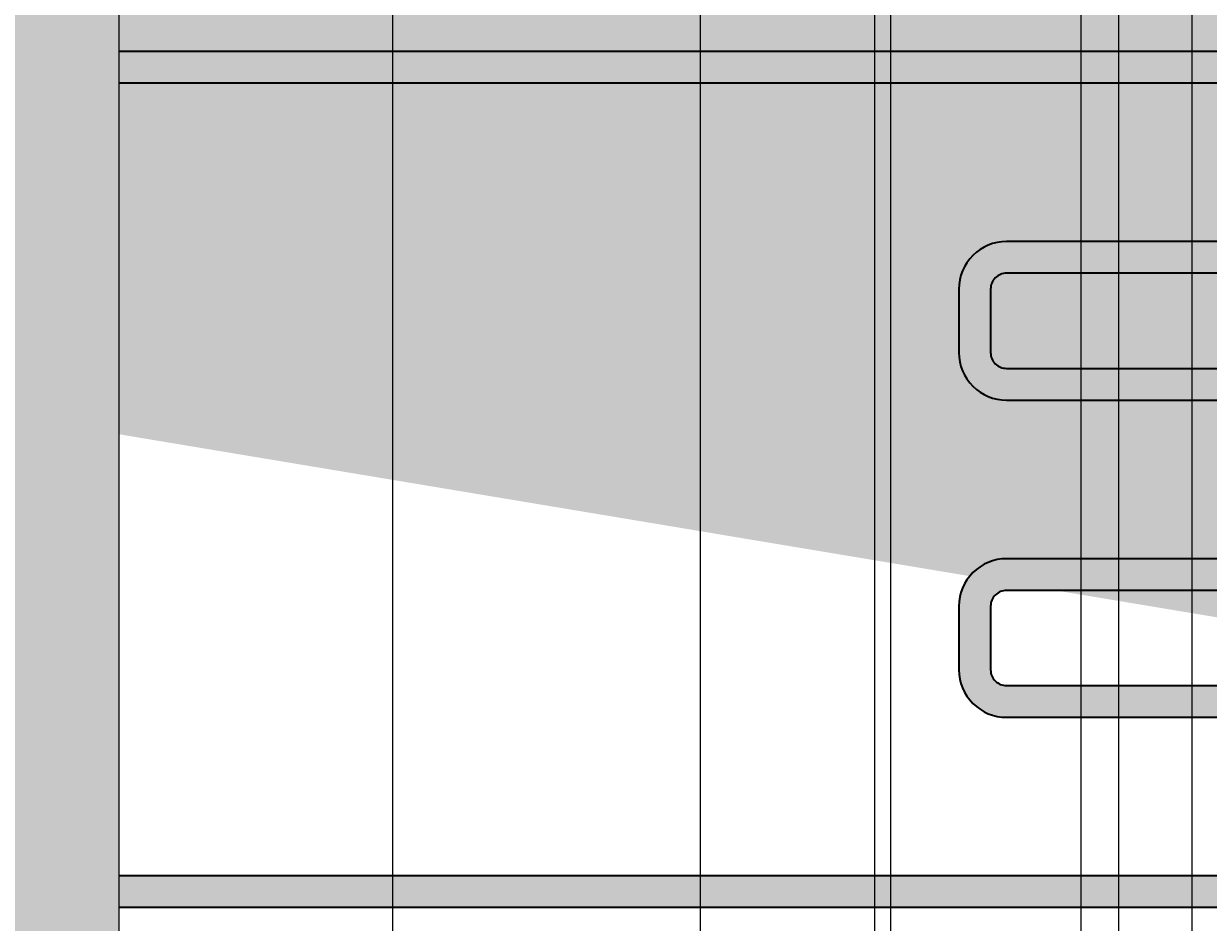
# Model space of a CAD drawing. Units: millimetres. Extents: x -22994 to 29398, y -19990 to 20176.
# Tile 44 of 135: x 99 to 136, y 96 to 124. Entities that reach past the tile are written whole.
import ezdxf

# ---------------------------------------------------------------- set-up
doc = ezdxf.new("R2010")
doc.units = ezdxf.units.MM
doc.header["$MEASUREMENT"] = 0
for name, color, linetype, lineweight in [('M-DIMS', 2, 'Continuous', 18), ('M-EQPM', 7, 'Continuous', 25), ('M-EQPM-PATT', 7, 'Continuous', 18), ('M-PIPE', 7, 'Continuous', 35)]:
    doc.layers.add(name, color=color, linetype=linetype, lineweight=lineweight)
doc.styles.get("Standard").update_dxf_attribs({"font": 'arial.ttf'})
doc.dimstyles.get("Standard").update_dxf_attribs({"dimtxt": 0.18, "dimasz": 10000, "dimexe": 0.18, "dimexo": 0.0625, "dimgap": 0.09, "dimtad": 0, "dimtih": 1, "dimtoh": 1, "dimdec": 0, "dimzin": 0, "dimdsep": 46, "dimtxsty": 'Standard', "dimcen": 0.09, "dimadec": 0, "dimazin": 0, "dimtfac": 1, "dimtdec": 0, "dimtofl": 0, "dimtmove": 0, "dimatfit": 3, "dimfxl": 1, "dimtolj": 1, "dimtzin": 0, "dimlwd": 30, "dimarcsym": 0})

# ---------------------------------------------------------------- blocks, each defined once
blk = doc.blocks.new('*D2')
at = {"layer": 'Defpoints', "color": 0, "transparency": 16777216}
for p in [(6.677, 10.271), (290.852, 10.271), (290.852, -5.079)]:
    blk.add_point(p, dxfattribs=at)
at = {"layer": 'M-DIMS', "color": 0, "lineweight": -2, "transparency": 16777216}
for p, q in [((6.677, 10.209), (6.677, -5.259)), ((290.852, 10.209), (290.852, -5.259))]:
    blk.add_line(p, q, dxfattribs=at)
at = {"layer": 'M-DIMS', "color": 0, "lineweight": 30, "transparency": 16777216}
for p, q in [((-9993.323, -5.079), (-19993.323, -5.079)), ((10290.852, -5.079), (20290.852, -5.079))]:
    blk.add_line(p, q, dxfattribs=at)
at = {"layer": 'M-DIMS', "color": 0, "transparency": 16777216}
for points in [[(-9993.323, 1661.588), (-9993.323, -1671.745), (6.677, -5.079)], [(10290.852, 1661.588), (10290.852, -1671.745), (290.852, -5.079)]]:
    blk.add_solid(points, dxfattribs=at)
at = {"layer": 'M-DIMS', "color": 0, "transparency": 16777216, "insert": (148.765, -5.079), "char_height": 0.18, "attachment_point": 5}
blk.add_mtext('\\A1;284.2', dxfattribs=at)
blk = doc.blocks.new('*D3')
at = {"layer": 'Defpoints', "color": 0, "transparency": 16777216}
for p in [(110.265, 204.165), (110.265, 176.366), (95.833, 127.967)]:
    blk.add_point(p, dxfattribs=at)
at = {"layer": 'M-DIMS', "color": 0, "lineweight": -2, "transparency": 16777216}
for p, q in [((95.833, 128.03), (95.833, 204.345)), ((110.265, 176.429), (110.265, 204.345))]:
    blk.add_line(p, q, dxfattribs=at)
at = {"layer": 'M-DIMS', "color": 0, "lineweight": 30, "transparency": 16777216}
for p, q in [((-9904.167, 204.165), (-19904.167, 204.165)), ((10110.265, 204.165), (20110.265, 204.165))]:
    blk.add_line(p, q, dxfattribs=at)
at = {"layer": 'M-DIMS', "color": 0, "transparency": 16777216}
for points in [[(-9904.167, 1870.832), (-9904.167, -1462.501), (95.833, 204.165)], [(10110.265, 1870.832), (10110.265, -1462.501), (110.265, 204.165)]]:
    blk.add_solid(points, dxfattribs=at)
at = {"layer": 'M-DIMS', "color": 0, "transparency": 16777216, "insert": (103.049, 204.165), "char_height": 0.18, "attachment_point": 5}
blk.add_mtext('\\A1;14.432', dxfattribs=at)
blk = doc.blocks.new('*D4')
at = {"layer": 'Defpoints', "color": 0, "transparency": 16777216}
for p in [(116.265, 204.165), (110.265, 176.366), (116.265, 176.366)]:
    blk.add_point(p, dxfattribs=at)
at = {"layer": 'M-DIMS', "color": 0, "lineweight": -2, "transparency": 16777216}
for p, q in [((110.265, 176.429), (110.265, 204.345)), ((116.265, 176.429), (116.265, 204.345))]:
    blk.add_line(p, q, dxfattribs=at)
at = {"layer": 'M-DIMS', "color": 0, "lineweight": 30, "transparency": 16777216}
for p, q in [((-9889.735, 204.165), (-19889.735, 204.165)), ((10116.265, 204.165), (20116.265, 204.165))]:
    blk.add_line(p, q, dxfattribs=at)
at = {"layer": 'M-DIMS', "color": 0, "transparency": 16777216}
for points in [[(-9889.735, 1870.832), (-9889.735, -1462.501), (110.265, 204.165)], [(10116.265, 1870.832), (10116.265, -1462.501), (116.265, 204.165)]]:
    blk.add_solid(points, dxfattribs=at)
at = {"layer": 'M-DIMS', "color": 0, "transparency": 16777216, "insert": (113.265, 204.165), "char_height": 0.18, "attachment_point": 5}
blk.add_mtext('\\A1;6', dxfattribs=at)
blk = doc.blocks.new('*D5')
at = {"layer": 'Defpoints', "color": 0, "transparency": 16777216}
for p in [(181.265, 204.165), (116.265, 176.366), (181.265, 176.366)]:
    blk.add_point(p, dxfattribs=at)
at = {"layer": 'M-DIMS', "color": 0, "lineweight": -2, "transparency": 16777216}
for p, q in [((116.265, 176.429), (116.265, 204.345)), ((181.265, 176.429), (181.265, 204.345))]:
    blk.add_line(p, q, dxfattribs=at)
at = {"layer": 'M-DIMS', "color": 0, "lineweight": 30, "transparency": 16777216}
for p, q in [((-9883.735, 204.165), (-19883.735, 204.165)), ((10181.265, 204.165), (20181.265, 204.165))]:
    blk.add_line(p, q, dxfattribs=at)
at = {"layer": 'M-DIMS', "color": 0, "transparency": 16777216}
for points in [[(-9883.735, 1870.832), (-9883.735, -1462.501), (116.265, 204.165)], [(10181.265, 1870.832), (10181.265, -1462.501), (181.265, 204.165)]]:
    blk.add_solid(points, dxfattribs=at)
at = {"layer": 'M-DIMS', "color": 0, "transparency": 16777216, "insert": (148.765, 204.165), "char_height": 0.18, "attachment_point": 5}
blk.add_mtext('\\A1;65', dxfattribs=at)
blk = doc.blocks.new('*D6')
at = {"layer": 'Defpoints', "color": 0, "transparency": 16777216}
for p in [(187.265, 204.165), (181.265, 176.366), (187.265, 176.366)]:
    blk.add_point(p, dxfattribs=at)
at = {"layer": 'M-DIMS', "color": 0, "lineweight": -2, "transparency": 16777216}
for p, q in [((181.265, 176.429), (181.265, 204.345)), ((187.265, 176.429), (187.265, 204.345))]:
    blk.add_line(p, q, dxfattribs=at)
at = {"layer": 'M-DIMS', "color": 0, "lineweight": 30, "transparency": 16777216}
for p, q in [((-9818.735, 204.165), (-19818.735, 204.165)), ((10187.265, 204.165), (20187.265, 204.165))]:
    blk.add_line(p, q, dxfattribs=at)
at = {"layer": 'M-DIMS', "color": 0, "transparency": 16777216}
for points in [[(-9818.735, 1870.832), (-9818.735, -1462.501), (181.265, 204.165)], [(10187.265, 1870.832), (10187.265, -1462.501), (187.265, 204.165)]]:
    blk.add_solid(points, dxfattribs=at)
at = {"layer": 'M-DIMS', "color": 0, "transparency": 16777216, "insert": (184.265, 204.165), "char_height": 0.18, "attachment_point": 5}
blk.add_mtext('\\A1;6', dxfattribs=at)
blk = doc.blocks.new('*D7')
at = {"layer": 'Defpoints', "color": 0, "transparency": 16777216}
for p in [(201.697, 204.165), (187.265, 176.366), (201.697, 127.967)]:
    blk.add_point(p, dxfattribs=at)
at = {"layer": 'M-DIMS', "color": 0, "lineweight": -2, "transparency": 16777216}
for p, q in [((187.265, 176.429), (187.265, 204.345)), ((201.697, 128.03), (201.697, 204.345))]:
    blk.add_line(p, q, dxfattribs=at)
at = {"layer": 'M-DIMS', "color": 0, "lineweight": 30, "transparency": 16777216}
for p, q in [((-9812.735, 204.165), (-19812.735, 204.165)), ((10201.697, 204.165), (20201.697, 204.165))]:
    blk.add_line(p, q, dxfattribs=at)
at = {"layer": 'M-DIMS', "color": 0, "transparency": 16777216}
for points in [[(-9812.735, 1870.832), (-9812.735, -1462.501), (187.265, 204.165)], [(10201.697, 1870.832), (10201.697, -1462.501), (201.697, 204.165)]]:
    blk.add_solid(points, dxfattribs=at)
at = {"layer": 'M-DIMS', "color": 0, "transparency": 16777216, "insert": (194.481, 204.165), "char_height": 0.18, "attachment_point": 5}
blk.add_mtext('\\A1;14.432', dxfattribs=at)
blk = doc.blocks.new('*D8')
at = {"layer": 'Defpoints', "color": 0, "transparency": 16777216}
for p in [(227.648, 204.165), (227.648, 146.73), (201.697, 127.967)]:
    blk.add_point(p, dxfattribs=at)
at = {"layer": 'M-DIMS', "color": 0, "lineweight": -2, "transparency": 16777216}
for p, q in [((201.697, 128.03), (201.697, 204.345)), ((227.648, 146.792), (227.648, 204.345))]:
    blk.add_line(p, q, dxfattribs=at)
at = {"layer": 'M-DIMS', "color": 0, "lineweight": 30, "transparency": 16777216}
for p, q in [((-9798.303, 204.165), (-19798.303, 204.165)), ((10227.648, 204.165), (20227.648, 204.165))]:
    blk.add_line(p, q, dxfattribs=at)
at = {"layer": 'M-DIMS', "color": 0, "transparency": 16777216}
for points in [[(-9798.303, 1870.832), (-9798.303, -1462.501), (201.697, 204.165)], [(10227.648, 1870.832), (10227.648, -1462.501), (227.648, 204.165)]]:
    blk.add_solid(points, dxfattribs=at)
at = {"layer": 'M-DIMS', "color": 0, "transparency": 16777216, "insert": (214.673, 204.165), "char_height": 0.18, "attachment_point": 5}
blk.add_mtext('\\A1;25.95', dxfattribs=at)
blk = doc.blocks.new('*D9')
at = {"layer": 'Defpoints', "color": 0, "transparency": 16777216}
for p in [(187.265, 176.366), (306.202, 176.366), (290.852, 10.271)]:
    blk.add_point(p, dxfattribs=at)
at = {"layer": 'M-DIMS', "color": 0, "lineweight": 30, "transparency": 16777216}
for p, q in [((306.202, 10176.366), (306.202, 20176.366)), ((306.202, -9989.729), (306.202, -19989.729))]:
    blk.add_line(p, q, dxfattribs=at)
at = {"layer": 'M-DIMS', "color": 0, "lineweight": -2, "transparency": 16777216}
for p, q in [((187.327, 176.366), (306.382, 176.366)), ((290.915, 10.271), (306.382, 10.271))]:
    blk.add_line(p, q, dxfattribs=at)
at = {"layer": 'M-DIMS', "color": 0, "transparency": 16777216}
for points in [[(-1360.465, 10176.366), (1972.869, 10176.366), (306.202, 176.366)], [(-1360.465, -9989.729), (1972.869, -9989.729), (306.202, 10.271)]]:
    blk.add_solid(points, dxfattribs=at)
at = {"layer": 'M-DIMS', "color": 0, "transparency": 16777216, "insert": (306.202, 93.319), "char_height": 0.18, "attachment_point": 5}
blk.add_mtext('\\A1;166.1', dxfattribs=at)
blk = doc.blocks.new('*D10')
at = {"layer": 'Defpoints', "color": 0, "transparency": 16777216}
for p in [(125.65, 136.071), (133.346, 136.071), (133.346, -5.079)]:
    blk.add_point(p, dxfattribs=at)
at = {"layer": 'M-DIMS', "color": 0, "lineweight": -2, "transparency": 16777216}
for p, q in [((125.65, 136.009), (125.65, -5.259)), ((133.346, 136.009), (133.346, -5.259))]:
    blk.add_line(p, q, dxfattribs=at)
at = {"layer": 'M-DIMS', "color": 0, "lineweight": 30, "transparency": 16777216}
for p, q in [((-9874.35, -5.079), (-19874.35, -5.079)), ((10133.346, -5.079), (20133.346, -5.079))]:
    blk.add_line(p, q, dxfattribs=at)
at = {"layer": 'M-DIMS', "color": 0, "transparency": 16777216}
for points in [[(-9874.35, 1661.588), (-9874.35, -1671.745), (125.65, -5.079)], [(10133.346, 1661.588), (10133.346, -1671.745), (133.346, -5.079)]]:
    blk.add_solid(points, dxfattribs=at)
at = {"layer": 'M-DIMS', "color": 0, "transparency": 16777216, "insert": (129.498, -5.079), "char_height": 0.18, "attachment_point": 5}
blk.add_mtext('\\A1;7.696', dxfattribs=at)
blk = doc.blocks.new('*D11')
at = {"layer": 'Defpoints', "color": 0, "transparency": 16777216}
for p in [(133.346, 136.071), (135.65, 136.071), (135.65, -5.079)]:
    blk.add_point(p, dxfattribs=at)
at = {"layer": 'M-DIMS', "color": 0, "lineweight": -2, "transparency": 16777216}
for p, q in [((133.346, 136.009), (133.346, -5.259)), ((135.65, 136.009), (135.65, -5.259))]:
    blk.add_line(p, q, dxfattribs=at)
at = {"layer": 'M-DIMS', "color": 0, "lineweight": 30, "transparency": 16777216}
for p, q in [((-9866.654, -5.079), (-19866.654, -5.079)), ((10135.65, -5.079), (20135.65, -5.079))]:
    blk.add_line(p, q, dxfattribs=at)
at = {"layer": 'M-DIMS', "color": 0, "transparency": 16777216}
for points in [[(-9866.654, 1661.588), (-9866.654, -1671.745), (133.346, -5.079)], [(10135.65, 1661.588), (10135.65, -1671.745), (135.65, -5.079)]]:
    blk.add_solid(points, dxfattribs=at)
at = {"layer": 'M-DIMS', "color": 0, "transparency": 16777216, "insert": (134.498, -5.079), "char_height": 0.18, "attachment_point": 5}
blk.add_mtext('\\A1;2.304', dxfattribs=at)
blk = doc.blocks.new('*D12')
at = {"layer": 'Defpoints', "color": 0, "transparency": 16777216}
for p in [(135.65, 136.071), (145.65, 136.071), (145.65, -5.079)]:
    blk.add_point(p, dxfattribs=at)
at = {"layer": 'M-DIMS', "color": 0, "lineweight": -2, "transparency": 16777216}
for p, q in [((135.65, 136.009), (135.65, -5.259)), ((145.65, 136.009), (145.65, -5.259))]:
    blk.add_line(p, q, dxfattribs=at)
at = {"layer": 'M-DIMS', "color": 0, "lineweight": 30, "transparency": 16777216}
for p, q in [((-9864.35, -5.079), (-19864.35, -5.079)), ((10145.65, -5.079), (20145.65, -5.079))]:
    blk.add_line(p, q, dxfattribs=at)
at = {"layer": 'M-DIMS', "color": 0, "transparency": 16777216}
for points in [[(-9864.35, 1661.588), (-9864.35, -1671.745), (135.65, -5.079)], [(10145.65, 1661.588), (10145.65, -1671.745), (145.65, -5.079)]]:
    blk.add_solid(points, dxfattribs=at)
at = {"layer": 'M-DIMS', "color": 0, "transparency": 16777216, "insert": (140.65, -5.079), "char_height": 0.18, "attachment_point": 5}
blk.add_mtext('\\A1;10', dxfattribs=at)
blk = doc.blocks.new('*D13')
at = {"layer": 'Defpoints', "color": 0, "transparency": 16777216}
for p in [(145.65, 136.071), (155.65, 136.071), (155.65, -5.079)]:
    blk.add_point(p, dxfattribs=at)
at = {"layer": 'M-DIMS', "color": 0, "lineweight": -2, "transparency": 16777216}
for p, q in [((145.65, 136.009), (145.65, -5.259)), ((155.65, 136.009), (155.65, -5.259))]:
    blk.add_line(p, q, dxfattribs=at)
at = {"layer": 'M-DIMS', "color": 0, "lineweight": 30, "transparency": 16777216}
for p, q in [((-9854.35, -5.079), (-19854.35, -5.079)), ((10155.65, -5.079), (20155.65, -5.079))]:
    blk.add_line(p, q, dxfattribs=at)
at = {"layer": 'M-DIMS', "color": 0, "transparency": 16777216}
for points in [[(-9854.35, 1661.588), (-9854.35, -1671.745), (145.65, -5.079)], [(10155.65, 1661.588), (10155.65, -1671.745), (155.65, -5.079)]]:
    blk.add_solid(points, dxfattribs=at)
at = {"layer": 'M-DIMS', "color": 0, "transparency": 16777216, "insert": (150.65, -5.079), "char_height": 0.18, "attachment_point": 5}
blk.add_mtext('\\A1;10', dxfattribs=at)
blk = doc.blocks.new('*D14')
at = {"layer": 'Defpoints', "color": 0, "transparency": 16777216}
for p in [(155.65, 136.071), (165.65, 136.071), (165.65, -5.079)]:
    blk.add_point(p, dxfattribs=at)
at = {"layer": 'M-DIMS', "color": 0, "lineweight": -2, "transparency": 16777216}
for p, q in [((155.65, 136.009), (155.65, -5.259)), ((165.65, 136.009), (165.65, -5.259))]:
    blk.add_line(p, q, dxfattribs=at)
at = {"layer": 'M-DIMS', "color": 0, "lineweight": 30, "transparency": 16777216}
for p, q in [((-9844.35, -5.079), (-19844.35, -5.079)), ((10165.65, -5.079), (20165.65, -5.079))]:
    blk.add_line(p, q, dxfattribs=at)
at = {"layer": 'M-DIMS', "color": 0, "transparency": 16777216}
for points in [[(-9844.35, 1661.588), (-9844.35, -1671.745), (155.65, -5.079)], [(10165.65, 1661.588), (10165.65, -1671.745), (165.65, -5.079)]]:
    blk.add_solid(points, dxfattribs=at)
at = {"layer": 'M-DIMS', "color": 0, "transparency": 16777216, "insert": (160.65, -5.079), "char_height": 0.18, "attachment_point": 5}
blk.add_mtext('\\A1;10', dxfattribs=at)
blk = doc.blocks.new('*D15')
at = {"layer": 'Defpoints', "color": 0, "transparency": 16777216}
for p in [(173.346, 154.788), (173.346, 136.071), (306.202, 136.071)]:
    blk.add_point(p, dxfattribs=at)
at = {"layer": 'M-DIMS', "color": 0, "lineweight": 30, "transparency": 16777216}
for p, q in [((306.202, 10154.788), (306.202, 20154.788)), ((306.202, -9863.929), (306.202, -19863.929))]:
    blk.add_line(p, q, dxfattribs=at)
at = {"layer": 'M-DIMS', "color": 0, "lineweight": -2, "transparency": 16777216}
for p, q in [((173.408, 154.788), (306.382, 154.788)), ((173.408, 136.071), (306.382, 136.071))]:
    blk.add_line(p, q, dxfattribs=at)
at = {"layer": 'M-DIMS', "color": 0, "transparency": 16777216}
for points in [[(-1360.465, 10154.788), (1972.869, 10154.788), (306.202, 154.788)], [(-1360.465, -9863.929), (1972.869, -9863.929), (306.202, 136.071)]]:
    blk.add_solid(points, dxfattribs=at)
at = {"layer": 'M-DIMS', "color": 0, "transparency": 16777216, "insert": (306.202, 145.43), "char_height": 0.18, "attachment_point": 5}
blk.add_mtext('\\A1;18.717', dxfattribs=at)
blk = doc.blocks.new('*D16')
at = {"layer": 'Defpoints', "color": 0, "transparency": 16777216}
for p in [(120.17, 204.165), (110.466, 48.035), (120.17, 48.035)]:
    blk.add_point(p, dxfattribs=at)
at = {"layer": 'M-DIMS', "color": 0, "lineweight": -2, "transparency": 16777216}
for p, q in [((110.466, 48.097), (110.466, 204.345)), ((120.17, 48.097), (120.17, 204.345))]:
    blk.add_line(p, q, dxfattribs=at)
at = {"layer": 'M-DIMS', "color": 0, "lineweight": 30, "transparency": 16777216}
for p, q in [((-9889.534, 204.165), (-19889.534, 204.165)), ((10120.17, 204.165), (20120.17, 204.165))]:
    blk.add_line(p, q, dxfattribs=at)
at = {"layer": 'M-DIMS', "color": 0, "transparency": 16777216}
for points in [[(-9889.534, 1870.832), (-9889.534, -1462.501), (110.466, 204.165)], [(10120.17, 1870.832), (10120.17, -1462.501), (120.17, 204.165)]]:
    blk.add_solid(points, dxfattribs=at)
at = {"layer": 'M-DIMS', "color": 0, "transparency": 16777216, "insert": (115.318, 204.165), "char_height": 0.18, "attachment_point": 5}
blk.add_mtext('\\A1;9.704', dxfattribs=at)
blk = doc.blocks.new('*D17')
at = {"layer": 'Defpoints', "color": 0, "transparency": 16777216}
for p in [(126.17, 204.165), (120.17, 48.035), (126.17, 48.035)]:
    blk.add_point(p, dxfattribs=at)
at = {"layer": 'M-DIMS', "color": 0, "lineweight": -2, "transparency": 16777216}
for p, q in [((120.17, 48.097), (120.17, 204.345)), ((126.17, 48.097), (126.17, 204.345))]:
    blk.add_line(p, q, dxfattribs=at)
at = {"layer": 'M-DIMS', "color": 0, "lineweight": 30, "transparency": 16777216}
for p, q in [((-9879.83, 204.165), (-19879.83, 204.165)), ((10126.17, 204.165), (20126.17, 204.165))]:
    blk.add_line(p, q, dxfattribs=at)
at = {"layer": 'M-DIMS', "color": 0, "transparency": 16777216}
for points in [[(-9879.83, 1870.832), (-9879.83, -1462.501), (120.17, 204.165)], [(10126.17, 1870.832), (10126.17, -1462.501), (126.17, 204.165)]]:
    blk.add_solid(points, dxfattribs=at)
at = {"layer": 'M-DIMS', "color": 0, "transparency": 16777216, "insert": (123.17, 204.165), "char_height": 0.18, "attachment_point": 5}
blk.add_mtext('\\A1;6', dxfattribs=at)
blk = doc.blocks.new('*D18')
at = {"layer": 'Defpoints', "color": 0, "transparency": 16777216}
for p in [(132.17, 204.165), (126.17, 48.035), (132.17, 48.035)]:
    blk.add_point(p, dxfattribs=at)
at = {"layer": 'M-DIMS', "color": 0, "lineweight": -2, "transparency": 16777216}
for p, q in [((126.17, 48.097), (126.17, 204.345)), ((132.17, 48.097), (132.17, 204.345))]:
    blk.add_line(p, q, dxfattribs=at)
at = {"layer": 'M-DIMS', "color": 0, "lineweight": 30, "transparency": 16777216}
for p, q in [((-9873.83, 204.165), (-19873.83, 204.165)), ((10132.17, 204.165), (20132.17, 204.165))]:
    blk.add_line(p, q, dxfattribs=at)
at = {"layer": 'M-DIMS', "color": 0, "transparency": 16777216}
for points in [[(-9873.83, 1870.832), (-9873.83, -1462.501), (126.17, 204.165)], [(10132.17, 1870.832), (10132.17, -1462.501), (132.17, 204.165)]]:
    blk.add_solid(points, dxfattribs=at)
at = {"layer": 'M-DIMS', "color": 0, "transparency": 16777216, "insert": (129.17, 204.165), "char_height": 0.18, "attachment_point": 5}
blk.add_mtext('\\A1;6', dxfattribs=at)
blk = doc.blocks.new('*D19')
at = {"layer": 'Defpoints', "color": 0, "transparency": 16777216}
for p in [(138.17, 204.165), (132.17, 48.035), (138.17, 48.035)]:
    blk.add_point(p, dxfattribs=at)
at = {"layer": 'M-DIMS', "color": 0, "lineweight": -2, "transparency": 16777216}
for p, q in [((132.17, 48.097), (132.17, 204.345)), ((138.17, 48.097), (138.17, 204.345))]:
    blk.add_line(p, q, dxfattribs=at)
at = {"layer": 'M-DIMS', "color": 0, "lineweight": 30, "transparency": 16777216}
for p, q in [((-9867.83, 204.165), (-19867.83, 204.165)), ((10138.17, 204.165), (20138.17, 204.165))]:
    blk.add_line(p, q, dxfattribs=at)
at = {"layer": 'M-DIMS', "color": 0, "transparency": 16777216}
for points in [[(-9867.83, 1870.832), (-9867.83, -1462.501), (132.17, 204.165)], [(10138.17, 1870.832), (10138.17, -1462.501), (138.17, 204.165)]]:
    blk.add_solid(points, dxfattribs=at)
at = {"layer": 'M-DIMS', "color": 0, "transparency": 16777216, "insert": (135.17, 204.165), "char_height": 0.18, "attachment_point": 5}
blk.add_mtext('\\A1;6', dxfattribs=at)
blk = doc.blocks.new('*D20')
at = {"layer": 'Defpoints', "color": 0, "transparency": 16777216}
for p in [(144.17, 204.165), (138.17, 48.035), (144.17, 48.035)]:
    blk.add_point(p, dxfattribs=at)
at = {"layer": 'M-DIMS', "color": 0, "lineweight": -2, "transparency": 16777216}
for p, q in [((138.17, 48.097), (138.17, 204.345)), ((144.17, 48.097), (144.17, 204.345))]:
    blk.add_line(p, q, dxfattribs=at)
at = {"layer": 'M-DIMS', "color": 0, "lineweight": 30, "transparency": 16777216}
for p, q in [((-9861.83, 204.165), (-19861.83, 204.165)), ((10144.17, 204.165), (20144.17, 204.165))]:
    blk.add_line(p, q, dxfattribs=at)
at = {"layer": 'M-DIMS', "color": 0, "transparency": 16777216}
for points in [[(-9861.83, 1870.832), (-9861.83, -1462.501), (138.17, 204.165)], [(10144.17, 1870.832), (10144.17, -1462.501), (144.17, 204.165)]]:
    blk.add_solid(points, dxfattribs=at)
at = {"layer": 'M-DIMS', "color": 0, "transparency": 16777216, "insert": (141.17, 204.165), "char_height": 0.18, "attachment_point": 5}
blk.add_mtext('\\A1;6', dxfattribs=at)
blk = doc.blocks.new('*D21')
at = {"layer": 'Defpoints', "color": 0, "transparency": 16777216}
for p in [(149.116, 204.165), (144.17, 48.035), (149.116, 48.035)]:
    blk.add_point(p, dxfattribs=at)
at = {"layer": 'M-DIMS', "color": 0, "lineweight": -2, "transparency": 16777216}
for p, q in [((144.17, 48.097), (144.17, 204.345)), ((149.116, 48.097), (149.116, 204.345))]:
    blk.add_line(p, q, dxfattribs=at)
at = {"layer": 'M-DIMS', "color": 0, "lineweight": 30, "transparency": 16777216}
for p, q in [((-9855.83, 204.165), (-19855.83, 204.165)), ((10149.116, 204.165), (20149.116, 204.165))]:
    blk.add_line(p, q, dxfattribs=at)
at = {"layer": 'M-DIMS', "color": 0, "transparency": 16777216}
for points in [[(-9855.83, 1870.832), (-9855.83, -1462.501), (144.17, 204.165)], [(10149.116, 1870.832), (10149.116, -1462.501), (149.116, 204.165)]]:
    blk.add_solid(points, dxfattribs=at)
at = {"layer": 'M-DIMS', "color": 0, "transparency": 16777216, "insert": (146.643, 204.165), "char_height": 0.18, "attachment_point": 5}
blk.add_mtext('\\A1;4.945', dxfattribs=at)
blk = doc.blocks.new('*D22')
at = {"layer": 'Defpoints', "color": 0, "transparency": 16777216}
for p in [(149.116, 30.99), (155.116, 30.99), (155.116, -5.079)]:
    blk.add_point(p, dxfattribs=at)
at = {"layer": 'M-DIMS', "color": 0, "lineweight": -2, "transparency": 16777216}
for p, q in [((149.116, 30.927), (149.116, -5.259)), ((155.116, 30.927), (155.116, -5.259))]:
    blk.add_line(p, q, dxfattribs=at)
at = {"layer": 'M-DIMS', "color": 0, "lineweight": 30, "transparency": 16777216}
for p, q in [((-9850.884, -5.079), (-19850.884, -5.079)), ((10155.116, -5.079), (20155.116, -5.079))]:
    blk.add_line(p, q, dxfattribs=at)
at = {"layer": 'M-DIMS', "color": 0, "transparency": 16777216}
for points in [[(-9850.884, 1661.588), (-9850.884, -1671.745), (149.116, -5.079)], [(10155.116, 1661.588), (10155.116, -1671.745), (155.116, -5.079)]]:
    blk.add_solid(points, dxfattribs=at)
at = {"layer": 'M-DIMS', "color": 0, "transparency": 16777216, "insert": (152.116, -5.079), "char_height": 0.18, "attachment_point": 5}
blk.add_mtext('\\A1;6', dxfattribs=at)
blk = doc.blocks.new('*D23')
at = {"layer": 'Defpoints', "color": 0, "transparency": 16777216}
for p in [(155.116, 30.99), (161.116, 30.99), (161.116, -5.079)]:
    blk.add_point(p, dxfattribs=at)
at = {"layer": 'M-DIMS', "color": 0, "lineweight": -2, "transparency": 16777216}
for p, q in [((155.116, 30.927), (155.116, -5.259)), ((161.116, 30.927), (161.116, -5.259))]:
    blk.add_line(p, q, dxfattribs=at)
at = {"layer": 'M-DIMS', "color": 0, "lineweight": 30, "transparency": 16777216}
for p, q in [((-9844.884, -5.079), (-19844.884, -5.079)), ((10161.116, -5.079), (20161.116, -5.079))]:
    blk.add_line(p, q, dxfattribs=at)
at = {"layer": 'M-DIMS', "color": 0, "transparency": 16777216}
for points in [[(-9844.884, 1661.588), (-9844.884, -1671.745), (155.116, -5.079)], [(10161.116, 1661.588), (10161.116, -1671.745), (161.116, -5.079)]]:
    blk.add_solid(points, dxfattribs=at)
at = {"layer": 'M-DIMS', "color": 0, "transparency": 16777216, "insert": (158.116, -5.079), "char_height": 0.18, "attachment_point": 5}
blk.add_mtext('\\A1;6', dxfattribs=at)
blk = doc.blocks.new('*D24')
at = {"layer": 'Defpoints', "color": 0, "transparency": 16777216}
for p in [(161.116, 30.99), (166.439, 30.99), (166.439, -5.079)]:
    blk.add_point(p, dxfattribs=at)
at = {"layer": 'M-DIMS', "color": 0, "lineweight": -2, "transparency": 16777216}
for p, q in [((161.116, 30.927), (161.116, -5.259)), ((166.439, 30.927), (166.439, -5.259))]:
    blk.add_line(p, q, dxfattribs=at)
at = {"layer": 'M-DIMS', "color": 0, "lineweight": 30, "transparency": 16777216}
for p, q in [((-9838.884, -5.079), (-19838.884, -5.079)), ((10166.439, -5.079), (20166.439, -5.079))]:
    blk.add_line(p, q, dxfattribs=at)
at = {"layer": 'M-DIMS', "color": 0, "transparency": 16777216}
for points in [[(-9838.884, 1661.588), (-9838.884, -1671.745), (161.116, -5.079)], [(10166.439, 1661.588), (10166.439, -1671.745), (166.439, -5.079)]]:
    blk.add_solid(points, dxfattribs=at)
at = {"layer": 'M-DIMS', "color": 0, "transparency": 16777216, "insert": (163.777, -5.079), "char_height": 0.18, "attachment_point": 5}
blk.add_mtext('\\A1;5.323', dxfattribs=at)
blk = doc.blocks.new('*D25')
at = {"layer": 'Defpoints', "color": 0, "transparency": 16777216}
for p in [(166.439, 30.99), (172.439, 30.99), (172.439, -5.079)]:
    blk.add_point(p, dxfattribs=at)
at = {"layer": 'M-DIMS', "color": 0, "lineweight": -2, "transparency": 16777216}
for p, q in [((166.439, 30.927), (166.439, -5.259)), ((172.439, 30.927), (172.439, -5.259))]:
    blk.add_line(p, q, dxfattribs=at)
at = {"layer": 'M-DIMS', "color": 0, "lineweight": 30, "transparency": 16777216}
for p, q in [((-9833.561, -5.079), (-19833.561, -5.079)), ((10172.439, -5.079), (20172.439, -5.079))]:
    blk.add_line(p, q, dxfattribs=at)
at = {"layer": 'M-DIMS', "color": 0, "transparency": 16777216}
for points in [[(-9833.561, 1661.588), (-9833.561, -1671.745), (166.439, -5.079)], [(10172.439, 1661.588), (10172.439, -1671.745), (172.439, -5.079)]]:
    blk.add_solid(points, dxfattribs=at)
at = {"layer": 'M-DIMS', "color": 0, "transparency": 16777216, "insert": (169.439, -5.079), "char_height": 0.18, "attachment_point": 5}
blk.add_mtext('\\A1;6', dxfattribs=at)
blk = doc.blocks.new('*D26')
at = {"layer": 'Defpoints', "color": 0, "transparency": 16777216}
for p in [(172.439, 30.99), (178.439, 30.99), (178.439, -5.079)]:
    blk.add_point(p, dxfattribs=at)
at = {"layer": 'M-DIMS', "color": 0, "lineweight": -2, "transparency": 16777216}
for p, q in [((172.439, 30.927), (172.439, -5.259)), ((178.439, 30.927), (178.439, -5.259))]:
    blk.add_line(p, q, dxfattribs=at)
at = {"layer": 'M-DIMS', "color": 0, "lineweight": 30, "transparency": 16777216}
for p, q in [((-9827.561, -5.079), (-19827.561, -5.079)), ((10178.439, -5.079), (20178.439, -5.079))]:
    blk.add_line(p, q, dxfattribs=at)
at = {"layer": 'M-DIMS', "color": 0, "transparency": 16777216}
for points in [[(-9827.561, 1661.588), (-9827.561, -1671.745), (172.439, -5.079)], [(10178.439, 1661.588), (10178.439, -1671.745), (178.439, -5.079)]]:
    blk.add_solid(points, dxfattribs=at)
at = {"layer": 'M-DIMS', "color": 0, "transparency": 16777216, "insert": (175.439, -5.079), "char_height": 0.18, "attachment_point": 5}
blk.add_mtext('\\A1;6', dxfattribs=at)
blk = doc.blocks.new('*D27')
at = {"layer": 'Defpoints', "color": 0, "transparency": 16777216}
for p in [(178.439, 30.99), (188.117, 30.99), (188.117, -5.079)]:
    blk.add_point(p, dxfattribs=at)
at = {"layer": 'M-DIMS', "color": 0, "lineweight": -2, "transparency": 16777216}
for p, q in [((178.439, 30.927), (178.439, -5.259)), ((188.117, 30.927), (188.117, -5.259))]:
    blk.add_line(p, q, dxfattribs=at)
at = {"layer": 'M-DIMS', "color": 0, "lineweight": 30, "transparency": 16777216}
for p, q in [((-9821.561, -5.079), (-19821.561, -5.079)), ((10188.117, -5.079), (20188.117, -5.079))]:
    blk.add_line(p, q, dxfattribs=at)
at = {"layer": 'M-DIMS', "color": 0, "transparency": 16777216}
for points in [[(-9821.561, 1661.588), (-9821.561, -1671.745), (178.439, -5.079)], [(10188.117, 1661.588), (10188.117, -1671.745), (188.117, -5.079)]]:
    blk.add_solid(points, dxfattribs=at)
at = {"layer": 'M-DIMS', "color": 0, "transparency": 16777216, "insert": (183.278, -5.079), "char_height": 0.18, "attachment_point": 5}
blk.add_mtext('\\A1;9.679', dxfattribs=at)
blk = doc.blocks.new('*D28')
at = {"layer": 'Defpoints', "color": 0, "transparency": 16777216}
for p in [(188.117, 48.035), (306.202, 48.035), (188.117, 30.99)]:
    blk.add_point(p, dxfattribs=at)
at = {"layer": 'M-DIMS', "color": 0, "lineweight": 30, "transparency": 16777216}
for p, q in [((306.202, 10048.035), (306.202, 20048.035)), ((306.202, -9969.01), (306.202, -19969.01))]:
    blk.add_line(p, q, dxfattribs=at)
at = {"layer": 'M-DIMS', "color": 0, "lineweight": -2, "transparency": 16777216}
for p, q in [((188.18, 48.035), (306.382, 48.035)), ((188.18, 30.99), (306.382, 30.99))]:
    blk.add_line(p, q, dxfattribs=at)
at = {"layer": 'M-DIMS', "color": 0, "transparency": 16777216}
for points in [[(-1360.465, 10048.035), (1972.869, 10048.035), (306.202, 48.035)], [(-1360.465, -9969.01), (1972.869, -9969.01), (306.202, 30.99)]]:
    blk.add_solid(points, dxfattribs=at)
at = {"layer": 'M-DIMS', "color": 0, "transparency": 16777216, "insert": (306.202, 39.512), "char_height": 0.18, "attachment_point": 5}
blk.add_mtext('\\A1;17.045', dxfattribs=at)
blk = doc.blocks.new('*D29')
at = {"layer": 'Defpoints', "color": 0, "transparency": 16777216}
for p in [(36.801, 80.045), (64.03, 80.045)]:
    blk.add_point(p, dxfattribs=at)
at = {"layer": 'M-DIMS', "color": 0, "lineweight": -2, "transparency": 16777216}
for p, q in [((50.325, 80.045), (50.505, 80.045)), ((50.415, 79.955), (50.415, 80.135))]:
    blk.add_line(p, q, dxfattribs=at)
at = {"layer": 'M-DIMS', "color": 0, "lineweight": 30, "transparency": 16777216}
blk.add_line((20064.03, 80.03), (10064.03, 80.038), dxfattribs=at)
at = {"layer": 'M-DIMS', "color": 0, "transparency": 16777216}
blk.add_solid([(10064.031, 1746.704), (10064.028, -1586.629), (64.03, 80.045)], dxfattribs=at)
at = {"layer": 'M-DIMS', "color": 0, "transparency": 16777216, "insert": (20064.521, 80.03), "char_height": 0.18, "attachment_point": 5}
blk.add_mtext('\\A1;∅27.23', dxfattribs=at)
blk = doc.blocks.new('*D36')
at = {"layer": 'Defpoints', "color": 0, "transparency": 16777216}
for p in [(46.39, 31.303), (46.387, 26.593)]:
    blk.add_point(p, dxfattribs=at)
at = {"layer": 'M-DIMS', "color": 0, "lineweight": 30, "transparency": 16777216}
for p, q in [((57.15, 20031.301), (51.77, 10031.302)), ((10057.15, 20031.301), (57.15, 20031.301))]:
    blk.add_line(p, q, dxfattribs=at)
at = {"layer": 'M-DIMS', "color": 0, "lineweight": -2, "transparency": 16777216}
for p, q in [((46.299, 28.948), (46.479, 28.948)), ((46.389, 28.858), (46.389, 29.038))]:
    blk.add_line(p, q, dxfattribs=at)
at = {"layer": 'M-DIMS', "color": 0, "transparency": 16777216}
blk.add_solid([(-1614.896, 10032.199), (1718.436, 10030.405), (46.39, 31.303)], dxfattribs=at)
at = {"layer": 'M-DIMS', "color": 0, "transparency": 16777216, "insert": (10057.554, 20031.301), "char_height": 0.18, "attachment_point": 5}
blk.add_mtext('\\A1;∅4.71', dxfattribs=at)
blk = doc.blocks.new('*D37')
at = {"layer": 'Defpoints', "color": 0, "transparency": 16777216}
for p in [(54.834, 118.615), (59.494, 118.614)]:
    blk.add_point(p, dxfattribs=at)
at = {"layer": 'M-DIMS', "color": 0, "lineweight": -2, "transparency": 16777216}
for p, q in [((57.074, 118.614), (57.254, 118.614)), ((57.164, 118.524), (57.164, 118.704))]:
    blk.add_line(p, q, dxfattribs=at)
at = {"layer": 'M-DIMS', "color": 0, "lineweight": 30, "transparency": 16777216}
blk.add_line((20059.493, 116.253), (10059.494, 117.434), dxfattribs=at)
at = {"layer": 'M-DIMS', "color": 0, "transparency": 16777216}
blk.add_solid([(10059.69, 1784.1), (10059.297, -1549.233), (59.494, 118.614)], dxfattribs=at)
at = {"layer": 'M-DIMS', "color": 0, "transparency": 16777216, "insert": (20059.985, 116.253), "char_height": 0.18, "attachment_point": 5}
blk.add_mtext('\\A1;∅4.659', dxfattribs=at)

msp = doc.modelspace()

# ---------------------------------------------------------------- hatches: boundary and pattern name
at = {"layer": 'M-EQPM-PATT'}
h = msp.add_hatch(color=256, dxfattribs=at)
h.set_gradient(color1=(205, 32, 39), color2=(205, 32, 39), tint=1)
h.paths.add_polyline_path([(116.2647, 150.3662), (116.2647, 170.3662), (116.2647, 176.3662), (110.2647, 176.3662), (110.2647, 152.0276), (95.8327, 127.967), (95.8327, 16.6063), (201.6967, 16.6063), (201.6967, 127.967), (187.2647, 152.0276), (187.2647, 176.3662), (181.2647, 176.3662), (181.2647, 170.3662), (181.2647, 150.3662), (195.6967, 126.3055), (195.6967, 22.6063), (101.8327, 22.6063), (101.8327, 126.3055)])
h.paths.add_polyline_path([(185.2208, 88.6347), (101.8327, 88.6347), (101.8327, 87.6347), (182.8066, 87.6347), (178.7313, 83.5594), (195.6967, 83.5594), (195.6967, 84.5594), (181.1455, 84.5594)], flags=17)
h.paths.add_polyline_path([(95.8327, 88.6347), (60.9779, 88.6347, -0.0228552), (61.7178, 87.6347), (95.8327, 87.6347)])
h.paths.add_polyline_path([(215.6212, 86.5189), (215.6212, 80.5999), (220.5095, 83.5594)])
h.paths.add_polyline_path([(215.6212, 84.5594), (201.6967, 84.5594), (201.6967, 83.5594), (215.6212, 83.5594)])
h.paths.add_polyline_path([(225.3978, 86.5189), (220.5095, 83.5594), (225.3978, 80.5999)])
h.paths.add_polyline_path([(231.6256, 84.5594), (225.3978, 84.5594), (225.3978, 83.5594), (231.6256, 83.5594)])
h = msp.add_hatch(color=256, dxfattribs=at)
h.set_gradient(color1=(34, 52, 110), color2=(41, 49, 137), tint=1, name='CYLINDER')
h.paths.add_polyline_path([(101.8327, 123.6277), (101.8327, 122.6277), (176.8123, 122.6277, -0.4142136), (178.3123, 121.1277), (178.3123, 119.1277, -0.4142136), (176.8123, 117.6277), (129.8123, 117.6277, 0.4142136), (128.3123, 116.1277), (128.3123, 114.1277, 0.4142136), (129.8123, 112.6277), (176.8123, 112.6277, -0.4142136), (178.3123, 111.1277), (178.3123, 109.1277, -0.4142136), (176.8123, 107.6277), (129.8123, 107.6277, 0.4142136), (128.3123, 106.1277), (128.3123, 104.1277, 0.4142136), (129.8123, 102.6277), (176.8123, 102.6277, -0.4142136), (178.3123, 101.1277), (178.3123, 99.1277, -0.4142136), (176.8123, 97.6277), (101.8327, 97.6277), (101.8327, 96.6277), (176.8123, 96.6277, 0.4142136), (179.3123, 99.1277), (179.3123, 101.1277, 0.4142136), (176.8123, 103.6277), (129.8123, 103.6277, -0.4142136), (129.3123, 104.1277), (129.3123, 106.1277, -0.4142136), (129.8123, 106.6277), (176.8123, 106.6277, 0.4142136), (179.3123, 109.1277), (179.3123, 111.1277, 0.4142136), (176.8123, 113.6277), (129.8123, 113.6277, -0.4142136), (129.3123, 114.1277), (129.3123, 116.1277, -0.4142136), (129.8123, 116.6277), (176.8123, 116.6277, 0.4142136), (179.3123, 119.1277), (179.3123, 121.1277, 0.4142136), (176.8123, 123.6277)])
h.paths.add_polyline_path([(75.6657, 123.6277), (75.6657, 122.6277), (95.8327, 122.6277), (95.8327, 123.6277)])
h.paths.add_polyline_path([(51.0853, 122.6277, -0.0439182), (51.8797, 123.6277), (38.9157, 123.6277), (38.9157, 122.6277)])
h.paths.add_polyline_path([(95.8327, 96.6277), (95.8327, 97.6277), (22.2694, 97.6277, 0.4142136), (20.7694, 96.1277), (20.7694, 89.8712, 0.4142136), (22.2694, 88.3712), (39.6435, 88.3712, -0.024152), (40.4967, 89.3712), (23.2694, 89.3712, -0.4142136), (21.7694, 90.8712), (21.7694, 95.1277, -0.4142136), (23.2694, 96.6277)])
h.paths.add_polyline_path([(137.7248, 106.4435), (168.6853, 106.4435), (168.6853, 114.6864), (137.7248, 114.6864)], flags=25)

# ---------------------------------------------------------------- linework, layer by layer
at = {"layer": 'M-EQPM'}
msp.add_lwpolyline([(116.2647, 170.3662), (116.2647, 150.3662), (101.8327, 126.3055), (101.8327, 22.6063), (195.6967, 22.6063), (195.6967, 126.3055), (181.2647, 150.3662), (181.2647, 170.3662)], dxfattribs=at)
at = {"layer": 'M-PIPE'}
for points in [[(101.8327, 123.6277), (176.8123, 123.6277, -0.4142136), (179.3123, 121.1277), (179.3123, 119.1277, -0.4142136), (176.8123, 116.6277), (129.8123, 116.6277, 0.4142136), (129.3123, 116.1277), (129.3123, 114.1277, 0.4142136), (129.8123, 113.6277), (176.8123, 113.6277, -0.4142136), (179.3123, 111.1277), (179.3123, 109.1277, -0.4142136), (176.8123, 106.6277), (129.8123, 106.6277, 0.4142136), (129.3123, 106.1277), (129.3123, 104.1277, 0.4142136), (129.8123, 103.6277), (176.8123, 103.6277, -0.4142136), (179.3123, 101.1277), (179.3123, 99.1277, -0.4142136), (176.8123, 96.6277), (101.8327, 96.6277)], [(101.8327, 122.6277), (176.8123, 122.6277, -0.4142136), (178.3123, 121.1277), (178.3123, 119.1277, -0.4142136), (176.8123, 117.6277), (129.8123, 117.6277, 0.4142136), (128.3123, 116.1277), (128.3123, 114.1277, 0.4142136), (129.8123, 112.6277), (176.8123, 112.6277, -0.4142136), (178.3123, 111.1277), (178.3123, 109.1277, -0.4142136), (176.8123, 107.6277), (129.8123, 107.6277, 0.4142136), (128.3123, 106.1277), (128.3123, 104.1277, 0.4142136), (129.8123, 102.6277), (176.8123, 102.6277, -0.4142136), (178.3123, 101.1277), (178.3123, 99.1277, -0.4142136), (176.8123, 97.6277), (101.8327, 97.6277)]]:
    msp.add_lwpolyline(points, format="xyb", dxfattribs=at)

# ---------------------------------------------------------------- dimensions: what is measured, and where the dimension line sits
at = {"layer": 'M-DIMS'}
for base, p1, p2, override, picture, middle in [((306.202, 176.3662), (290.852, 10.2713), (187.2647, 176.3662), {"dimdec": 1, "dimlfac": 1, "dimrnd": 0, "dimzin": 0, "dimdsep": 46, "dimlunit": 2}, '*D9', (306.202, 93.3187)), ((306.202, 136.0713), (173.3459, 154.788), (173.3459, 136.0713), {"dimdec": 3, "dimlfac": 1, "dimrnd": 0, "dimzin": 0, "dimdsep": 46, "dimlunit": 2}, '*D15', (306.202, 145.4297)), ((306.202, 48.0349), (188.1175, 30.9895), (188.1175, 48.0349), {"dimdec": 3, "dimlfac": 1, "dimrnd": 0, "dimzin": 0, "dimdsep": 46, "dimlunit": 2}, '*D28', (306.202, 39.5122))]:
    dim = msp.add_linear_dim(base=base, p1=p1, p2=p2, angle=90, dimstyle='Standard', override=override, dxfattribs=at)
    dim.commit()
    dim.dimension.update_dxf_attribs({"geometry": picture, "text_midpoint": middle})
dim = msp.add_diameter_dim_2p(p1=(46.3875, 26.5934), p2=(46.39, 31.3035), dimstyle='Standard', override={"dimdec": 2, "dimlfac": 1, "dimrnd": 0, "dimzin": 0, "dimdsep": 46, "dimlunit": 2}, dxfattribs=at)
dim.commit()
dim.dimension.update_dxf_attribs({"geometry": '*D36', "text_midpoint": (10057.5542, 20031.3006), "dimtype": 163})
for base, p1, p2, override, picture, middle in [((110.2647, 204.1654), (95.8327, 127.967), (110.2647, 176.3662), {"dimdec": 3, "dimlfac": 1, "dimrnd": 0, "dimzin": 0, "dimdsep": 46, "dimlunit": 2}, '*D3', (103.0487, 204.1654)), ((116.2647, 204.1654), (110.2647, 176.3662), (116.2647, 176.3662), {"dimdec": 0, "dimlfac": 1, "dimrnd": 0, "dimzin": 0, "dimdsep": 46, "dimlunit": 2}, '*D4', (113.2647, 204.1654)), ((120.1702, 204.1654), (110.4658, 48.0349), (120.1702, 48.0349), {"dimdec": 3, "dimlfac": 1, "dimrnd": 0, "dimzin": 0, "dimdsep": 46, "dimlunit": 2}, '*D16', (115.318, 204.1654)), ((181.2647, 204.1654), (116.2647, 176.3662), (181.2647, 176.3662), {"dimdec": 0, "dimlfac": 1, "dimrnd": 0, "dimzin": 0, "dimdsep": 46, "dimlunit": 2}, '*D5', (148.7647, 204.1654)), ((126.1702, 204.1654), (120.1702, 48.0349), (126.1702, 48.0349), {"dimdec": 0, "dimlfac": 1, "dimrnd": 0, "dimzin": 0, "dimdsep": 46, "dimlunit": 2}, '*D17', (123.1702, 204.1654)), ((132.1702, 204.1654), (126.1702, 48.0349), (132.1702, 48.0349), {"dimdec": 0, "dimlfac": 1, "dimrnd": 0, "dimzin": 0, "dimdsep": 46, "dimlunit": 2}, '*D18', (129.1702, 204.1654)), ((138.1702, 204.1654), (132.1702, 48.0349), (138.1702, 48.0349), {"dimdec": 0, "dimlfac": 1, "dimrnd": 0, "dimzin": 0, "dimdsep": 46, "dimlunit": 2}, '*D19', (135.1702, 204.1654)), ((144.1702, 204.1654), (138.1702, 48.0349), (144.1702, 48.0349), {"dimdec": 0, "dimlfac": 1, "dimrnd": 0, "dimzin": 0, "dimdsep": 46, "dimlunit": 2}, '*D20', (141.1702, 204.1654)), ((149.11567, 204.16539), (144.17023, 48.03494), (149.11567, 48.03494), {"dimdec": 3, "dimlfac": 1, "dimrnd": 0, "dimzin": 0, "dimdsep": 46, "dimlunit": 2}, '*D21', (146.64295, 204.16539)), ((187.2647, 204.1654), (181.2647, 176.3662), (187.2647, 176.3662), {"dimdec": 0, "dimlfac": 1, "dimrnd": 0, "dimzin": 0, "dimdsep": 46, "dimlunit": 2}, '*D6', (184.2647, 204.1654)), ((201.6967, 204.1654), (187.2647, 176.3662), (201.6967, 127.967), {"dimdec": 3, "dimlfac": 1, "dimrnd": 0, "dimzin": 0, "dimdsep": 46, "dimlunit": 2}, '*D7', (194.4807, 204.1654)), ((227.6485, 204.1654), (201.6967, 127.967), (227.6485, 146.7296), {"dimdec": 2, "dimlfac": 1, "dimrnd": 0, "dimzin": 0, "dimdsep": 46, "dimlunit": 2}, '*D8', (214.6726, 204.1654)), ((290.852, -5.0787), (6.6773, 10.2713), (290.852, 10.2713), {"dimdec": 1, "dimlfac": 1, "dimrnd": 0, "dimzin": 0, "dimdsep": 46, "dimlunit": 2}, '*D2', (148.7647, -5.0787)), ((133.3459, -5.0787), (125.6498, 136.0713), (133.3459, 136.0713), {"dimdec": 3, "dimlfac": 1, "dimrnd": 0, "dimzin": 0, "dimdsep": 46, "dimlunit": 2}, '*D10', (129.4978, -5.0787)), ((135.6498, -5.0787), (133.3459, 136.0713), (135.6498, 136.0713), {"dimdec": 3, "dimlfac": 1, "dimrnd": 0, "dimzin": 0, "dimdsep": 46, "dimlunit": 2}, '*D11', (134.4978, -5.0787)), ((145.6498, -5.0787), (135.6498, 136.0713), (145.6498, 136.0713), {"dimdec": 0, "dimlfac": 1, "dimrnd": 0, "dimzin": 0, "dimdsep": 46, "dimlunit": 2}, '*D12', (140.6498, -5.0787)), ((155.6498, -5.0787), (145.6498, 136.0713), (155.6498, 136.0713), {"dimdec": 0, "dimlfac": 1, "dimrnd": 0, "dimzin": 0, "dimdsep": 46, "dimlunit": 2}, '*D13', (150.6498, -5.0787)), ((155.1157, -5.0787), (149.1157, 30.9895), (155.1157, 30.9895), {"dimdec": 0, "dimlfac": 1, "dimrnd": 0, "dimzin": 0, "dimdsep": 46, "dimlunit": 2}, '*D22', (152.1157, -5.0787)), ((161.1157, -5.0787), (155.1157, 30.9895), (161.1157, 30.9895), {"dimdec": 0, "dimlfac": 1, "dimrnd": 0, "dimzin": 0, "dimdsep": 46, "dimlunit": 2}, '*D23', (158.1157, -5.0787)), ((165.6498, -5.0787), (155.6498, 136.0713), (165.6498, 136.0713), {"dimdec": 0, "dimlfac": 1, "dimrnd": 0, "dimzin": 0, "dimdsep": 46, "dimlunit": 2}, '*D14', (160.6498, -5.0787)), ((166.4387, -5.0787), (161.1157, 30.9895), (166.4387, 30.9895), {"dimdec": 3, "dimlfac": 1, "dimrnd": 0, "dimzin": 0, "dimdsep": 46, "dimlunit": 2}, '*D24', (163.7772, -5.0787)), ((172.4387, -5.0787), (166.4387, 30.9895), (172.4387, 30.9895), {"dimdec": 0, "dimlfac": 1, "dimrnd": 0, "dimzin": 0, "dimdsep": 46, "dimlunit": 2}, '*D25', (169.4387, -5.0787)), ((178.4387, -5.0787), (172.4387, 30.9895), (178.4387, 30.9895), {"dimdec": 0, "dimlfac": 1, "dimrnd": 0, "dimzin": 0, "dimdsep": 46, "dimlunit": 2}, '*D26', (175.4387, -5.0787)), ((188.1175, -5.0787), (178.4387, 30.9895), (188.1175, 30.9895), {"dimdec": 3, "dimlfac": 1, "dimrnd": 0, "dimzin": 0, "dimdsep": 46, "dimlunit": 2}, '*D27', (183.2781, -5.0787))]:
    dim = msp.add_linear_dim(base=base, p1=p1, p2=p2, dimstyle='Standard', override=override, dxfattribs=at)
    dim.commit()
    dim.dimension.update_dxf_attribs({"geometry": picture, "text_midpoint": middle})
for p1, p2, override, picture, middle in [((54.8343, 118.6145), (59.4936, 118.614), {"dimdec": 3, "dimlfac": 1, "dimrnd": 0, "dimzin": 0, "dimdsep": 46, "dimlunit": 2}, '*D37', (20059.4934, 116.2531)), ((36.8006, 80.045), (64.0296, 80.045), {"dimdec": 2, "dimlfac": 1, "dimrnd": 0, "dimzin": 0, "dimdsep": 46, "dimlunit": 2}, '*D29', (20064.0296, 80.0303))]:
    dim = msp.add_diameter_dim_2p(p1=p1, p2=p2, dimstyle='Standard', override=override, dxfattribs=at)
    dim.commit()
    dim.dimension.update_dxf_attribs({"geometry": picture, "text_midpoint": middle})

doc.saveas('drawing.dxf')
